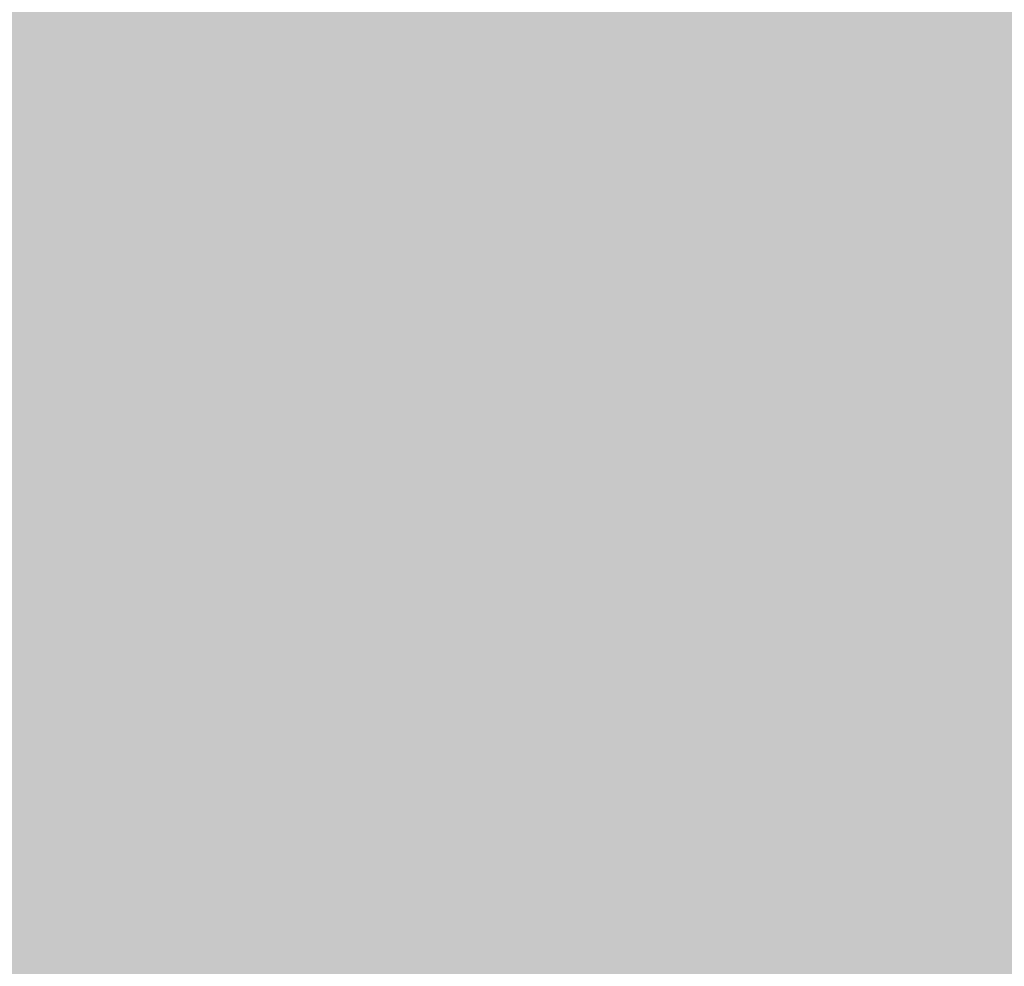
# Model space of a CAD drawing. Units: inches. Extents: x 2083 to 3317, y 1141 to 2115.
# Tile 137 of 256: x 3123.979 to 3126.132, y 1265.165 to 1267.234. Entities that reach past the tile are written whole.
import ezdxf

# ---------------------------------------------------------------- set-up
doc = ezdxf.new("R2010")
doc.units = ezdxf.units.IN
doc.layers.add('A-ANNO-DIMS', color=2, linetype='Continuous', lineweight=18)
doc.layers.add('A-WALL-PATT', color=251, linetype='Continuous', lineweight=13, true_color=0x636466)
doc.styles.get("Standard").update_dxf_attribs({"font": 'arial.ttf'})
doc.dimstyles.new('ISO-25', dxfattribs={"dimtxt": 12, "dimasz": 12, "dimexe": 1.25, "dimexo": 0.625, "dimtad": 1, "dimlunit": 3, "dimtxsty": 'Standard', "dimcen": 2.5, "dimadec": 0, "dimazin": 0, "dimtfac": 1, "dimtmove": 0, "dimatfit": 3, "dimfxl": 1, "dimarcsym": 0})

# ---------------------------------------------------------------- blocks, each defined once
blk = doc.blocks.new('*D26')
at = {"layer": 'A-ANNO-DIMS', "color": 0, "lineweight": -2, "transparency": 16777216}
for p, q in [((3088.9858, 1274.9151), (3088.9858, 1270.952)), ((3111.24, 1274.9151), (3111.24, 1270.952)), ((3076.9858, 1272.202), (2840.2624, 1272.202)), ((3111.24, 1272.202), (3088.9858, 1272.202)), ((3123.24, 1272.202), (3135.24, 1272.202))]:
    blk.add_line(p, q, dxfattribs=at)
at = {"layer": 'A-ANNO-DIMS', "color": 0, "transparency": 16777216}
for points in [[(3076.9858, 1274.202), (3076.9858, 1270.202), (3088.9858, 1272.202)], [(3123.24, 1274.202), (3123.24, 1270.202), (3111.24, 1272.202)]]:
    blk.add_solid(points, dxfattribs=at)
at = {"layer": 'Defpoints', "color": 0, "transparency": 16777216}
for p in [(3088.9858, 1275.5401), (3111.24, 1275.5401), (3088.9858, 1272.202)]:
    blk.add_point(p, dxfattribs=at)
at = {"layer": 'A-ANNO-DIMS', "color": 0, "transparency": 16777216, "insert": (2952.6241, 1279.0316), "char_height": 12, "attachment_point": 5}
blk.add_mtext('NIGHTSTAND 1\'-10 1/2" TYP.', dxfattribs=at)
blk = doc.blocks.new('*D27')
at = {"layer": 'A-ANNO-DIMS', "color": 0, "lineweight": -2, "transparency": 16777216}
for p, q in [((3114.5782, 1309.7943), (3114.5782, 1321.7943)), ((3111.865, 1297.7943), (3115.8282, 1297.7943)), ((3114.5782, 1297.7943), (3114.5782, 1275.5401)), ((3111.865, 1275.5401), (3115.8282, 1275.5401)), ((3114.5782, 1263.5401), (3114.5782, 1140.9886))]:
    blk.add_line(p, q, dxfattribs=at)
at = {"layer": 'A-ANNO-DIMS', "color": 0, "transparency": 16777216}
for points in [[(3112.5782, 1309.7943), (3116.5782, 1309.7943), (3114.5782, 1297.7943)], [(3112.5782, 1263.5401), (3116.5782, 1263.5401), (3114.5782, 1275.5401)]]:
    blk.add_solid(points, dxfattribs=at)
at = {"layer": 'Defpoints', "color": 0, "transparency": 16777216}
for p in [(3111.24, 1297.7943), (3111.24, 1275.5401), (3114.5782, 1275.5401)]:
    blk.add_point(p, dxfattribs=at)
at = {"layer": 'A-ANNO-DIMS', "color": 0, "transparency": 16777216, "insert": (3107.7485, 1196.2643), "char_height": 12, "attachment_point": 5, "rotation": 90}
blk.add_mtext('1\'-10 1/2" TYP.', dxfattribs=at)

msp = doc.modelspace()

# ---------------------------------------------------------------- hatches: boundary and pattern name
at = {"layer": 'A-WALL-PATT'}
h = msp.add_hatch(color=256, dxfattribs=at)
h.dxf.hatch_style = 1
h.paths.add_polyline_path([(3126.9598, 2020.7614), (2748.9598, 2020.7614), (2604.9598, 2020.7614), (2226.9598, 2020.7614), (2226.9598, 1702.7614), (2466.9598, 1702.7614), (2466.9598, 1582.7614), (2418.9598, 1582.7614), (2418.9598, 1477.7614), (2226.9598, 1477.7614), (2226.9598, 1263.2614), (2544.9598, 1263.2614), (2544.9598, 1411.7614), (2604.9598, 1411.7614), (2685.9598, 1411.7614), (2685.9598, 1420.7614), (2604.9598, 1420.7614), (2604.9598, 1573.7614), (2604.9598, 1702.7614), (2604.9598, 2011.7614), (2748.9598, 2011.7614), (2748.9598, 1702.7614), (2862.9598, 1702.7614), (2862.9598, 1621.7614), (2871.9598, 1621.7614), (2871.9598, 1702.7614), (2883.9598, 1702.7614), (2883.9598, 1706.9395, -0.026459), (2883.9598, 1711.7614), (2757.9598, 1711.7614), (2757.9598, 1807.7614), (2787.9598, 1807.7614), (2787.9598, 1812.2614), (2757.9598, 1812.2614), (2757.9598, 2011.7614), (2877.9598, 2011.7614), (2877.9598, 1812.2614), (2847.9598, 1812.2614), (2847.9598, 1807.7614), (2889.8357, 1807.7614), (2889.8357, 1812.2614), (2882.4598, 1812.2614), (2882.4598, 2011.7614), (3117.9598, 2011.7614), (3117.9598, 1812.2614), (2937.8357, 1812.2614), (2937.8357, 1807.7614), (2995.7098, 1807.7614), (2995.7098, 1796.1177), (3000.2098, 1796.1177), (3000.2098, 1807.7614), (3117.9598, 1807.7614), (3117.9598, 1711.7614), (3000.2098, 1711.7614), (3000.2098, 1760.1177), (2998.5727, 1760.1177, -0.020711), (2995.7098, 1760.1177), (2995.7098, 1711.7614), (2931.9598, 1711.7614), (2931.9598, 1702.7614), (3126.9598, 1702.7614)])
h.paths.add_polyline_path([(2471.4598, 2011.7614), (2471.4598, 1810.0114), (2462.7169, 1810.0114), (2462.7169, 1805.5114), (2505.9598, 1805.5114), (2505.9598, 1810.0114), (2475.9598, 1810.0114), (2475.9598, 2011.7614), (2595.9598, 2011.7614), (2595.9598, 1810.0114), (2565.9598, 1810.0114), (2565.9598, 1805.5114), (2595.9598, 1805.5114), (2595.9598, 1711.7614), (2235.9598, 1711.7614), (2235.9598, 1805.5114), (2353.7098, 1805.5114), (2353.7098, 1796.0542), (2358.2098, 1796.0542), (2358.2098, 1805.5114), (2414.7169, 1805.5114), (2414.7169, 1810.0114), (2235.9598, 1810.0114), (2235.9598, 2011.7614)], flags=16)
h.paths.add_polyline_path([(2270.2047, 1994.61), (2270.2047, 1970.61), (2246.2047, 1970.61), (2246.2047, 1994.61)], flags=0)
edge = h.paths.add_edge_path(flags=0)
edge.add_ellipse((2332.0274, 1899.7982), major_axis=(-3.043, 3.043), ratio=0.168252, start_angle=-161.3322, end_angle=-156.3071, ccw=False)
edge.add_ellipse((2333.082, 1898.7435), major_axis=(-1.0546, 1.0546), ratio=0.453532, start_angle=-123.371, end_angle=-94.1591)
edge = h.paths.add_edge_path(flags=0)
edge.add_ellipse((2332.0274, 1968.8763), major_axis=(3.043, 3.043), ratio=0.168252, start_angle=18.6678, end_angle=23.6929)
edge.add_spline(control_points=[(2332.9256, 1970.6911), (2332.2268, 1970.3361), (2330.8937, 1969.6589), (2328.4131, 1970.9321), (2327.2039, 1967.7487), (2324.7096, 1969.9556), (2322.5328, 1967.0124), (2320.0128, 1971.2958), (2317.6803, 1968.1578), (2316.0405, 1967.102), (2315.4269, 1966.8096)], knot_values=[0, 0, 0, 0, 2.267059, 4.324559, 6.685584, 8.878641, 11.121502, 14.300359, 17.755284, 19.732645, 19.732645, 19.732645, 19.732645], degree=3, periodic=0)
edge.add_ellipse((2332.0274, 1968.8763), major_axis=(3.043, 3.043), ratio=0.168252, start_angle=18.6678, end_angle=23.6929, ccw=False)
edge.add_ellipse((2333.082, 1969.9309), major_axis=(1.0546, 1.0546), ratio=0.453532, start_angle=56.629, end_angle=85.8409, ccw=False)
edge = h.paths.add_edge_path(flags=0)
edge.add_spline(control_points=[(2296.4283, 1967.9879), (2293.6278, 1965.3363), (2287.7036, 1959.7271), (2299.7439, 1949.9957), (2294.5326, 1935.6685), (2290.5732, 1920.6035), (2293.3941, 1909.9737), (2296.1854, 1904.9665)], knot_values=[0.099185, 0.099185, 0.099185, 0.099185, 0.345301, 0.619822, 0.982653, 1.386093, 1.810555, 1.810555, 1.810555, 1.810555], degree=3, periodic=0)
edge.add_spline(control_points=[(2296.1854, 1904.9665), (2297.3836, 1902.6193), (2298.001, 1901.9493), (2298.553, 1901.4682)], knot_values=[0.006246, 0.006246, 0.006246, 0.006246, 0.055476, 0.055476, 0.055476, 0.055476], degree=3, periodic=0)
edge.add_spline(control_points=[(2298.553, 1901.4682), (2297.2586, 1900.9232), (2295.2253, 1900.2321), (2293.0602, 1900.6142), (2292.1014, 1900.7884), (2292.0896, 1900.7906)], knot_values=[0.312835, 0.312835, 0.312835, 0.312835, 0.40178, 0.474987, 0.475903, 0.475903, 0.475903, 0.475903], degree=3, periodic=0)
edge.add_arc((2292.7936, 1904.6641), 3.937, 215.4209, 259.6982, ccw=False)
edge.add_spline(control_points=[(2289.5853, 1902.3823), (2289.4767, 1902.5351), (2289.3685, 1902.688), (2289.2609, 1902.8412)], knot_values=[0.102872, 0.102872, 0.102872, 0.102872, 0.116896, 0.116896, 0.116896, 0.116896], degree=3, periodic=0)
edge.add_spline(control_points=[(2289.2609, 1902.8412), (2288.6866, 1902.5502), (2287.64, 1902.0199), (2285.8813, 1901.874), (2283.853, 1901.5044), (2281.72, 1899.7105), (2278.467, 1899.4929), (2276.1571, 1901.8832), (2272.259, 1899.8041), (2267.7776, 1901.8432), (2262.2439, 1900.184), (2257.4149, 1901.7821), (2254.3184, 1900.7261), (2253.1783, 1900.3373)], knot_values=[0, 0, 0, 0, 1.907977, 3.477176, 5.261074, 7.972851, 11.680248, 13.717921, 16.939592, 22.789562, 27.502503, 33.595215, 37.145618, 37.145618, 37.145618, 37.145618], degree=3, periodic=0)
edge.add_line((2253.1783, 1900.3373), (2250.2442, 1902.8412))
edge.add_line((2250.2442, 1902.8412), (2250.2442, 1965.8333))
edge.add_line((2250.2442, 1965.8333), (2253.1783, 1968.3371))
edge.add_spline(control_points=[(2253.1783, 1968.3371), (2254.3184, 1967.9483), (2257.4149, 1966.8924), (2262.2439, 1968.4904), (2267.7776, 1966.8313), (2271.5267, 1968.5372), (2273.8759, 1967.8283), (2274.2067, 1967.7276)], knot_values=[0, 0, 0, 0, 0.09018, 0.244935, 0.364644, 0.513233, 0.537855, 0.537855, 0.537855, 0.537855], degree=3, periodic=0)
edge.add_arc((2274.3529, 1963.7933), 3.937, 72.0511, 92.1279, ccw=False)
edge.add_arc((2281.2969, 1985.23), 18.5963, 252.05113, 288.56572)
edge.add_arc((2292.3167, 1956.0289), 12.6461, 71.02679, 113.77822, ccw=False)
edge = h.paths.add_edge_path(flags=0)
edge.add_spline(control_points=[(2274.8994, 1951.8562), (2275.0662, 1951.6166), (2275.2327, 1951.3766), (2275.398, 1951.1359)], knot_values=[1.409916, 1.409916, 1.409916, 1.409916, 1.43159, 1.43159, 1.43159, 1.43159], degree=3, periodic=0)
edge.add_spline(control_points=[(2275.398, 1951.1359), (2275.7921, 1950.5619), (2276.1792, 1949.9838), (2276.5455, 1949.3971)], knot_values=[1.358238, 1.358238, 1.358238, 1.358238, 1.409916, 1.409916, 1.409916, 1.409916], degree=3, periodic=0)
edge.add_line((2276.5455, 1949.3971), (2277.4373, 1947.8622))
edge.add_spline(control_points=[(2277.4373, 1947.8622), (2276.3038, 1945.6731), (2274.6397, 1942.4269), (2274.6316, 1938.0939), (2272.7991, 1930.8515), (2274.3564, 1943.897), (2275.9477, 1947.9234), (2276.5455, 1949.3971)], knot_values=[0.005632, 0.005632, 0.005632, 0.005632, 0.186014, 0.266002, 0.357087, 0.59639, 0.739732, 0.739732, 0.739732, 0.739732], degree=3, periodic=0)
edge.add_spline(control_points=[(2276.5455, 1949.3971), (2276.1792, 1949.9838), (2275.7921, 1950.5619), (2275.398, 1951.1359)], knot_values=[1.358238, 1.358238, 1.358238, 1.358238, 1.409916, 1.409916, 1.409916, 1.409916], degree=3, periodic=0)
edge.add_spline(control_points=[(2275.398, 1951.1359), (2274.9425, 1950.0805), (2274.2078, 1948.0253), (2273.9346, 1944.8515), (2272.4685, 1937.6275), (2273.4662, 1945.6965), (2274.7006, 1951.0595), (2274.8994, 1951.8562)], knot_values=[0.104364, 0.104364, 0.104364, 0.104364, 0.189636, 0.269624, 0.36071, 0.600013, 0.644622, 0.644622, 0.644622, 0.644622], degree=3, periodic=0)
h.paths.add_polyline_path([(2269.1675, 1963.1276, -0.357527), (2268.1706, 1960.9764, -0.092561), (2268.1706, 1939.4363, -0.357527), (2269.1675, 1937.2851, -0.357527), (2267.0163, 1938.282, -0.164785), (2254.6856, 1938.282, -0.357527), (2252.5344, 1937.2851, -0.357527), (2253.5313, 1939.4363, -0.092561), (2253.5313, 1960.9764, -0.357527), (2252.5344, 1963.1276, -0.357527), (2254.6856, 1962.1307, -0.164785), (2267.0163, 1962.1307, -0.357527)], flags=0)
h.paths.add_polyline_path([(2248.8741, 1967.8018), (2248.8741, 1957.0277), (2249.4578, 1957.0277), (2249.4578, 1911.6468), (2248.8741, 1911.6468), (2248.8741, 1900.8727), (2246.5119, 1900.8727, 0.197327), (2244.1497, 1902.4569), (2244.1497, 1966.2176, 0.197327), (2246.5119, 1967.8018)], flags=0)
h.paths.add_polyline_path([(2269.1675, 1931.3893, -0.357527), (2268.1706, 1929.2381, -0.092561), (2268.1706, 1907.6981, -0.357527), (2269.1675, 1905.5469, -0.357527), (2267.0163, 1906.5438, -0.164785), (2254.6856, 1906.5438, -0.357527), (2252.5344, 1905.5469, -0.357527), (2253.5313, 1907.6981, -0.092561), (2253.5313, 1929.2381, -0.357527), (2252.5344, 1931.3893, -0.357527), (2254.6856, 1930.3925, -0.164785), (2267.0163, 1930.3925, -0.357527)], flags=0)
edge = h.paths.add_edge_path(flags=0)
edge.add_spline(control_points=[(2276.1969, 1906.7237), (2276.1681, 1909.0289), (2276.114, 1913.3719), (2270.5984, 1924.925), (2273.9052, 1919.0128), (2275.9217, 1916.2621), (2275.4746, 1912.4021), (2277.2579, 1910.3806), (2276.696, 1908.225), (2276.6462, 1906.813), (2276.6178, 1906.0084)], knot_values=[0, 0, 0, 0, 8.61026, 16.221274, 18.843057, 23.804898, 27.440828, 29.356102, 31.203478, 33.650687, 33.650687, 33.650687, 33.650687], degree=3, periodic=0)
edge.add_spline(control_points=[(2276.6178, 1906.0084), (2276.6233, 1905.6241), (2276.4977, 1904.6287), (2275.4418, 1903.8547), (2274.9373, 1903.0804), (2274.8591, 1902.8412)], knot_values=[0.156488, 0.156488, 0.156488, 0.156488, 0.184398, 0.231376, 0.250598, 0.250598, 0.250598, 0.250598], degree=3, periodic=0)
edge.add_line((2274.8591, 1902.8412), (2276.506, 1902.8412))
edge.add_spline(control_points=[(2276.506, 1902.8412), (2276.7883, 1903.0849), (2277.6651, 1904.1252), (2278.2495, 1904.3407), (2277.6539, 1908.5274), (2278.1557, 1906.2278), (2278.1005, 1905.2859), (2278.8467, 1904.069), (2277.8568, 1903.4149), (2277.8742, 1902.991), (2277.9036, 1902.8412)], knot_values=[0.059574, 0.059574, 0.059574, 0.059574, 0.080753, 0.103741, 0.16972, 0.176036, 0.207137, 0.240474, 0.262341, 0.27366, 0.27366, 0.27366, 0.27366], degree=3, periodic=0)
edge.add_line((2277.9036, 1902.8412), (2280.0298, 1902.8412))
edge.add_spline(control_points=[(2280.0298, 1902.8412), (2279.8882, 1903.0884), (2279.4993, 1903.9816), (2280.1523, 1905.9393), (2278.1036, 1909.6578), (2279.7624, 1907.1853), (2280.3279, 1904.8749), (2280.4851, 1903.4896), (2281.4633, 1903.2494), (2281.7583, 1902.9365), (2281.834, 1902.8412)], knot_values=[0.013856, 0.013856, 0.013856, 0.013856, 0.034874, 0.088867, 0.107879, 0.126738, 0.158714, 0.193757, 0.217487, 0.226722, 0.226722, 0.226722, 0.226722], degree=3, periodic=0)
edge.add_spline(control_points=[(2281.834, 1902.8412), (2281.7875, 1902.8267), (2281.647, 1902.783), (2281.3955, 1902.8595), (2281.0881, 1902.9852), (2280.7207, 1903.0609), (2280.3335, 1903.0257), (2280.1248, 1902.8989), (2280.0298, 1902.8412)], knot_values=[0, 0, 0, 0, 0.14413, 0.435517, 0.749276, 1.153046, 1.548371, 1.878348, 1.878348, 1.878348, 1.878348], degree=3, periodic=0)
edge.add_line((2280.0298, 1902.8412), (2277.9036, 1902.8412))
edge.add_spline(control_points=[(2277.9036, 1902.8412), (2277.8929, 1902.7959), (2277.8654, 1902.6796), (2277.6075, 1902.6875), (2277.2741, 1902.8007), (2276.8379, 1902.6198), (2276.5838, 1902.7893), (2276.506, 1902.8412)], knot_values=[0, 0, 0, 0, 0.127189, 0.326199, 0.628009, 1.24357, 1.515331, 1.515331, 1.515331, 1.515331], degree=3, periodic=0)
edge.add_line((2276.506, 1902.8412), (2274.8591, 1902.8412))
edge.add_spline(control_points=[(2274.8591, 1902.8412), (2274.8144, 1902.8986), (2274.7251, 1903.0134), (2274.4935, 1903.119), (2274.2443, 1902.9605), (2273.9371, 1903.1849), (2273.614, 1902.9831), (2273.4083, 1902.883), (2273.3223, 1902.8412)], knot_values=[0, 0, 0, 0, 0.21843, 0.436957, 0.687977, 0.990379, 1.398396, 1.69185, 1.69185, 1.69185, 1.69185], degree=3, periodic=0)
edge.add_spline(control_points=[(2273.3223, 1902.8412), (2273.6167, 1903.4457), (2274.274, 1904.5383), (2276.0272, 1904.5737), (2276.207, 1906.5836), (2276.1969, 1906.7237)], knot_values=[0.012227, 0.012227, 0.012227, 0.012227, 0.059472, 0.106218, 0.134458, 0.134458, 0.134458, 0.134458], degree=3, periodic=0)
h.paths.add_polyline_path([(2270.7761, 1897.7898), (2270.7761, 1873.7898), (2246.7761, 1873.7898), (2246.7761, 1897.7898)], flags=0)
h.paths.add_polyline_path([(2353.7098, 1760.0051), (2353.7098, 1760.0542), (2358.2098, 1760.0542, -0.033729)], flags=0)
h.paths.add_polyline_path([(2321.8191, 1737.5292), (2341.9953, 1737.5292, -0.414214), (2343.2033, 1736.3212), (2343.2033, 1721.0206, -0.414214), (2341.9953, 1719.8127), (2321.8191, 1719.8127, -0.414214), (2320.6112, 1721.0206), (2320.6112, 1736.3212, -0.414214)], flags=0)
h.paths.add_polyline_path([(2324.235, 1736.3212), (2339.5794, 1736.3212, -0.414214), (2341.9953, 1733.9053), (2341.9953, 1725.4497, -0.414214), (2339.5794, 1723.0338), (2333.6806, 1723.0338), (2333.8453, 1722.0455, -0.870646), (2335.4254, 1721.8259, -0.767327), (2333.9227, 1721.4232), (2331.291, 1721.4232, -0.767327), (2329.7883, 1721.8259, -0.870646), (2331.3684, 1722.0455), (2331.5331, 1723.0338), (2324.235, 1723.0338, -0.414214), (2321.8191, 1725.4497), (2321.8191, 1733.9053, -0.414214)], flags=0)
h.paths.add_polyline_path([(2570.4838, 1928.6154), (2589.6838, 1928.6154), (2590.1688, 1928.6154), (2590.1688, 1904.9934), (2570.4838, 1904.9934)], flags=0)
h.paths.add_polyline_path([(2574.4473, 1927.2638, -1), (2572.8288, 1927.2638, -1)], flags=0)
h.paths.add_polyline_path([(2573.0899, 1926.9409), (2573.925, 1927.776), (2574.1477, 1927.5533), (2573.3126, 1926.7182)], flags=0)
h.paths.add_polyline_path([(2578.7791, 1919.7296, -1), (2571.5917, 1919.7296, -1)], flags=0)
h.paths.add_polyline_path([(2578.3854, 1919.7296, -1), (2571.9854, 1919.7296, -1)], flags=0)
h.paths.add_polyline_path([(2331.5958, 1729.4762, -1), (2333.618, 1729.4762, -1)], flags=0)
h.paths.add_polyline_path([(2578.0342, 1927.2638, -1), (2576.4157, 1927.2638, -1)], flags=0)
h.paths.add_polyline_path([(2576.6889, 1927.5311), (2576.9116, 1927.7538), (2577.7467, 1926.9186), (2577.524, 1926.6959)], flags=0)
h.paths.add_polyline_path([(2578.1391, 1909.8595, -1), (2572.2317, 1909.8595, -1)], flags=0)
h.paths.add_polyline_path([(2577.7454, 1909.8595, -1), (2572.6254, 1909.8595, -1)], flags=0)
h.paths.add_polyline_path([(2583.7977, 1927.2638, -1), (2582.1792, 1927.2638, -1)], flags=0)
h.paths.add_polyline_path([(2582.7186, 1927.7538), (2583.5538, 1926.9186), (2583.3311, 1926.6959), (2582.4959, 1927.5311)], flags=0)
h.paths.add_polyline_path([(2582.4959, 1927.5311), (2582.7186, 1927.7538), (2583.5538, 1926.9186), (2583.3311, 1926.6959)], flags=0)
h.paths.add_polyline_path([(2587.7391, 1920.5296, -1), (2581.8317, 1920.5296, -1)], flags=0)
h.paths.add_polyline_path([(2587.3454, 1920.5296, -1), (2582.2254, 1920.5296, -1)], flags=0)
h.paths.add_polyline_path([(2587.3846, 1927.2638, -1), (2585.7661, 1927.2638, -1)], flags=0)
h.paths.add_polyline_path([(2586.082, 1926.9802), (2586.9172, 1927.8154), (2587.1399, 1927.5927), (2586.3047, 1926.7575)], flags=0)
h.paths.add_polyline_path([(2588.3791, 1910.6595, -1), (2581.1917, 1910.6595, -1)], flags=0)
h.paths.add_polyline_path([(2587.9854, 1910.6595, -1), (2581.5854, 1910.6595, -1)], flags=0)
h.paths.add_polyline_path([(2417.1677, 1729.4779), (2437.3439, 1729.4779, -0.414214), (2438.5519, 1728.2699), (2438.5519, 1712.9693, -0.414214), (2437.3439, 1711.7614), (2417.1677, 1711.7614, -0.414214), (2415.9598, 1712.9693), (2415.9598, 1728.2699, -0.414214)], flags=0)
h.paths.add_polyline_path([(2419.5836, 1728.2699), (2434.928, 1728.2699, -0.414214), (2437.3439, 1725.8541), (2437.3439, 1717.3984, -0.414214), (2434.928, 1714.9825), (2429.0292, 1714.9825), (2429.1939, 1713.9942, -0.870646), (2430.774, 1713.7746, -0.767327), (2429.2713, 1713.372), (2426.6396, 1713.372, -0.767327), (2425.1369, 1713.7746, -0.870646), (2426.717, 1713.9942), (2426.8817, 1714.9825), (2419.5836, 1714.9825, -0.414214), (2417.1677, 1717.3984), (2417.1677, 1725.8541, -0.414214)], flags=0)
h.paths.add_polyline_path([(2419.5836, 1728.2699), (2434.928, 1728.2699, -0.414214), (2437.3439, 1725.8541), (2437.3439, 1717.3984, -0.414214), (2434.928, 1714.9825), (2429.0292, 1714.9825), (2428.3581, 1719.009), (2427.5528, 1719.009), (2426.8817, 1714.9825), (2419.5836, 1714.9825, -0.414214), (2417.1677, 1717.3984), (2417.1677, 1725.8541, -0.414214)], flags=0)
h.paths.add_polyline_path([(2426.9444, 1721.4249, -1), (2428.9666, 1721.4249, -1)], flags=0)
h.paths.add_polyline_path([(2475.9598, 1702.7614), (2595.9598, 1702.7614), (2595.9598, 1582.7614), (2475.9598, 1582.7614)], flags=16)
h.paths.add_polyline_path([(2427.9598, 1573.7614), (2595.9598, 1573.7614), (2595.9598, 1468.7614), (2595.9598, 1420.7614), (2384.4598, 1420.7614), (2384.4598, 1468.7614), (2427.9598, 1468.7614)], flags=16)
h.paths.add_polyline_path([(2379.9598, 1468.7614), (2379.9598, 1420.7614), (2235.9598, 1420.7614), (2235.9598, 1468.7614)], flags=16)
h.paths.add_polyline_path([(2317.816, 1466.6958), (2337.9922, 1466.6958, -0.414214), (2339.2002, 1465.4878), (2339.2002, 1450.1872, -0.414214), (2337.9922, 1448.9792), (2317.816, 1448.9792, -0.414214), (2316.6081, 1450.1872), (2316.6081, 1465.4878, -0.414214)], flags=0)
h.paths.add_polyline_path([(2320.2319, 1465.4878), (2335.5763, 1465.4878, -0.414214), (2337.9922, 1463.0719), (2337.9922, 1454.6163, -0.414214), (2335.5763, 1452.2004), (2329.6775, 1452.2004), (2329.8422, 1451.212, -0.870646), (2331.4223, 1450.9925, -0.767327), (2329.9196, 1450.5898), (2327.2879, 1450.5898, -0.767327), (2325.7852, 1450.9925, -0.870646), (2327.3653, 1451.212), (2327.53, 1452.2004), (2320.2319, 1452.2004, -0.414214), (2317.816, 1454.6163), (2317.816, 1463.0719, -0.414214)], flags=0)
h.paths.add_polyline_path([(2320.2319, 1465.4878), (2335.5763, 1465.4878, -0.414214), (2337.9922, 1463.0719), (2337.9922, 1454.6163, -0.414214), (2335.5763, 1452.2004), (2329.6775, 1452.2004), (2329.0064, 1456.2269), (2328.2011, 1456.2269), (2327.53, 1452.2004), (2320.2319, 1452.2004, -0.414214), (2317.816, 1454.6163), (2317.816, 1463.0719, -0.414214)], flags=0)
h.paths.add_polyline_path([(2327.5926, 1458.6428, -1), (2329.6148, 1458.6428, -1)], flags=0)
h.paths.add_polyline_path([(2244.4117, 1433.3405), (2241.9209, 1433.3405, -0.414214), (2240.0179, 1435.2435), (2240.0179, 1440.9528, -0.414211), (2241.9209, 1442.8559), (2244.4117, 1442.8559, -1.976472)], flags=0)
h.paths.add_polyline_path([(2245.3569, 1434.3975, -0.414214), (2245.3569, 1441.7988, -2.144098)], flags=0)
h.paths.add_polyline_path([(2535.9598, 1416.2614), (2535.9598, 1272.2614), (2235.9598, 1272.2614), (2235.9598, 1416.2614)], flags=16)
h.paths.add_polyline_path([(2260.1196, 1384.2928), (2260.1196, 1362.0386), (2237.8654, 1362.0386), (2237.8654, 1384.2928)], flags=0)
edge = h.paths.add_edge_path(flags=0)
edge.add_line((2318.2518, 1362.0933), (2318.1458, 1362.001))
edge.add_ellipse((2317.4451, 1360.431), major_axis=(2.8216, 2.8216), ratio=0.168252, start_angle=18.6678, end_angle=20.9481, ccw=False)
edge.add_ellipse((2318.423, 1361.409), major_axis=(0.9779, 0.9779), ratio=0.453532, start_angle=56.629, end_angle=70.2262, ccw=False)
edge = h.paths.add_edge_path(flags=0)
edge.add_line((2319.1074, 1295.5711), (2319.015, 1295.6771))
edge.add_ellipse((2317.4451, 1296.3778), major_axis=(-2.8216, 2.8216), ratio=0.168252, start_angle=-161.3322, end_angle=-159.0519, ccw=False)
edge.add_ellipse((2318.423, 1295.3999), major_axis=(-0.9779, 0.9779), ratio=0.453532, start_angle=-123.371, end_angle=-109.7738)
edge = h.paths.add_edge_path(flags=0)
edge.add_spline(control_points=[(2284.2103, 1301.1702), (2284.5807, 1300.4447), (2284.8912, 1299.892), (2285.1596, 1299.461)], knot_values=[0.039066, 0.039066, 0.039066, 0.039066, 0.055476, 0.055476, 0.055476, 0.055476], degree=3, periodic=0)
edge.add_line((2285.1596, 1299.461), (2284.2103, 1301.1702))
edge = h.paths.add_edge_path(flags=0)
edge.add_line((2280.4125, 1297.298), (2283.37, 1297.0361))
edge.add_line((2283.37, 1297.0361), (2286.4057, 1297.9263))
edge.add_spline(control_points=[(2286.4057, 1297.9263), (2285.3055, 1297.4631), (2284.3448, 1297.1292), (2283.37, 1297.0361)], knot_values=[0.394369, 0.394369, 0.394369, 0.394369, 0.475903, 0.475903, 0.475903, 0.475903], degree=3, periodic=0)
edge.add_spline(control_points=[(2283.37, 1297.0361), (2283.2814, 1297.0277), (2282.3163, 1296.9573), (2281.3125, 1297.1345), (2280.4234, 1297.296), (2280.4125, 1297.298)], knot_values=[0.312835, 0.312835, 0.312835, 0.312835, 0.320246, 0.393453, 0.394369, 0.394369, 0.394369, 0.394369], degree=3, periodic=0)
edge = h.paths.add_edge_path(flags=0)
edge.add_line((2284.4356, 1359.6073), (2280.4463, 1355.328))
edge.add_line((2280.4463, 1355.328), (2279.58, 1351.0178))
edge.add_line((2279.58, 1351.0178), (2282.413, 1346.5804))
edge.add_spline(control_points=[(2282.413, 1346.5804), (2283.1533, 1345.5892), (2284.2529, 1344.0289), (2284.801, 1342.3872), (2284.9352, 1341.8055)], knot_values=[1.240098, 1.240098, 1.240098, 1.240098, 1.332892, 1.382712, 1.382712, 1.382712, 1.382712], degree=3, periodic=0)
edge.add_spline(control_points=[(2284.9352, 1341.8055), (2285.3191, 1340.1406), (2285.233, 1338.4092), (2284.9099, 1336.6541)], knot_values=[1.097484, 1.097484, 1.097484, 1.097484, 1.240098, 1.240098, 1.240098, 1.240098], degree=3, periodic=0)
edge.add_spline(control_points=[(2284.9099, 1336.6541), (2284.5868, 1334.899), (2284.0267, 1333.1203), (2283.4626, 1331.3606)], knot_values=[0.95487, 0.95487, 0.95487, 0.95487, 1.097484, 1.097484, 1.097484, 1.097484], degree=3, periodic=0)
edge.add_line((2283.4626, 1331.3606), (2281.8904, 1326.1534))
edge.add_line((2281.8904, 1326.1534), (2280.7563, 1321.0561))
edge.add_line((2280.7563, 1321.0561), (2280.2992, 1316.002))
edge.add_line((2280.2992, 1316.002), (2280.7159, 1310.9501))
edge.add_line((2280.7159, 1310.9501), (2282.0281, 1305.9721))
edge.add_line((2282.0281, 1305.9721), (2284.2103, 1301.1702))
edge.add_spline(control_points=[(2284.2103, 1301.1702), (2283.3407, 1302.7302), (2282.6119, 1304.3365), (2282.0281, 1305.9721)], knot_values=[0.099185, 0.099185, 0.099185, 0.099185, 0.241799, 0.241799, 0.241799, 0.241799], degree=3, periodic=0)
edge.add_spline(control_points=[(2282.0281, 1305.9721), (2281.4443, 1307.6078), (2281.0055, 1309.2728), (2280.7159, 1310.9501)], knot_values=[0.241799, 0.241799, 0.241799, 0.241799, 0.384413, 0.384413, 0.384413, 0.384413], degree=3, periodic=0)
edge.add_spline(control_points=[(2280.7159, 1310.9501), (2280.4332, 1312.5876), (2280.2894, 1314.277), (2280.2989, 1315.962), (2280.2992, 1316.002)], knot_values=[0.384413, 0.384413, 0.384413, 0.384413, 0.523647, 0.527028, 0.527028, 0.527028, 0.527028], degree=3, periodic=0)
edge.add_spline(control_points=[(2280.2992, 1316.002), (2280.3123, 1317.687), (2280.4779, 1319.3679), (2280.7563, 1321.0561)], knot_values=[0.527028, 0.527028, 0.527028, 0.527028, 0.669642, 0.669642, 0.669642, 0.669642], degree=3, periodic=0)
edge.add_spline(control_points=[(2280.7563, 1321.0561), (2281.0346, 1322.7443), (2281.4259, 1324.4396), (2281.8904, 1326.1534)], knot_values=[0.669642, 0.669642, 0.669642, 0.669642, 0.812256, 0.812256, 0.812256, 0.812256], degree=3, periodic=0)
edge.add_spline(control_points=[(2281.8904, 1326.1534), (2282.2644, 1327.5333), (2282.7879, 1329.2618), (2283.3528, 1331.0178), (2283.4626, 1331.3606)], knot_values=[0.812256, 0.812256, 0.812256, 0.812256, 0.927087, 0.95487, 0.95487, 0.95487, 0.95487], degree=3, periodic=0)
edge.add_line((2283.4626, 1331.3606), (2284.9099, 1336.6541))
edge.add_line((2284.9099, 1336.6541), (2284.9352, 1341.8055))
edge.add_line((2284.9352, 1341.8055), (2282.413, 1346.5804))
edge.add_spline(control_points=[(2282.413, 1346.5804), (2281.2751, 1348.1038), (2280.0784, 1349.5703), (2279.58, 1351.0178)], knot_values=[1.382712, 1.382712, 1.382712, 1.382712, 1.525326, 1.525326, 1.525326, 1.525326], degree=3, periodic=0)
edge.add_spline(control_points=[(2279.58, 1351.0178), (2279.4433, 1351.4147), (2279.1363, 1352.8569), (2279.7352, 1354.2904), (2280.4463, 1355.328)], knot_values=[1.525326, 1.525326, 1.525326, 1.525326, 1.564439, 1.667941, 1.667941, 1.667941, 1.667941], degree=3, periodic=0)
edge.add_spline(control_points=[(2280.4463, 1355.328), (2281.4261, 1356.7578), (2282.9308, 1358.1826), (2284.4356, 1359.6073)], knot_values=[1.667941, 1.667941, 1.667941, 1.667941, 1.810555, 1.810555, 1.810555, 1.810555], degree=3, periodic=0)
edge.add_arc((2280.6231, 1348.5182), 11.7262, 71.02679, 113.77822)
edge.add_arc((2270.4049, 1375.5952), 17.2436, 252.05113, 288.56572, ccw=False)
edge.add_arc((2263.966, 1355.7178), 3.6506, 72.0511, 92.1279)
edge.add_arc((2263.966, 1355.7178), 3.6506, 92.1279, 177.9851)
edge.add_spline(control_points=[(2260.3176, 1355.8462), (2260.2604, 1354.2207), (2260.5513, 1350.1865), (2262.9993, 1346.7663), (2264.4727, 1344.649)], knot_values=[1.43159, 1.43159, 1.43159, 1.43159, 1.564144, 1.770695, 1.770695, 1.770695, 1.770695], degree=3, periodic=0)
edge.add_line((2264.4727, 1344.649), (2264.9356, 1343.9825))
edge.add_spline(control_points=[(2263.801, 1340.2481), (2263.8432, 1340.5141), (2264.0672, 1341.7565), (2264.5127, 1343.0025), (2264.935, 1343.9811)], knot_values=[0.53657, 0.53657, 0.53657, 0.53657, 0.559349, 0.644622, 0.644622, 0.644622, 0.644622], degree=3, periodic=0)
edge.add_spline(control_points=[(2264.935, 1343.9811), (2265.1178, 1343.715), (2265.2989, 1343.4479), (2265.4768, 1343.1794)], knot_values=[1.384077, 1.384077, 1.384077, 1.384077, 1.409916, 1.409916, 1.409916, 1.409916], degree=3, periodic=0)
edge.add_spline(control_points=[(2265.4768, 1343.1794), (2265.6546, 1342.9108), (2265.8293, 1342.6408), (2265.9991, 1342.3688)], knot_values=[1.358238, 1.358238, 1.358238, 1.358238, 1.384077, 1.384077, 1.384077, 1.384077], degree=3, periodic=0)
edge.add_line((2265.9991, 1342.3688), (2266.826, 1340.9455))
edge.add_spline(control_points=[(2266.826, 1340.9455), (2268.8944, 1337.0897), (2271.3982, 1325.843), (2270.5162, 1310.5686), (2275.9194, 1301.8606), (2277.7895, 1299.1994)], knot_values=[0.116896, 0.116896, 0.116896, 0.116896, 0.472987, 1.050969, 1.313793, 1.313793, 1.313793, 1.313793], degree=3, periodic=0)
edge.add_spline(control_points=[(2277.7895, 1299.1994), (2277.8394, 1299.1285), (2277.8894, 1299.0575), (2277.9396, 1298.9866)], knot_values=[0.109884, 0.109884, 0.109884, 0.109884, 0.116896, 0.116896, 0.116896, 0.116896], degree=3, periodic=0)
edge.add_line((2277.9396, 1298.9866), (2277.7888, 1299.1991))
edge.add_spline(control_points=[(2277.7888, 1299.1991), (2277.2566, 1298.9294), (2276.2864, 1298.4379), (2275.0394, 1298.3344), (2274.3833, 1298.2389), (2274.2153, 1298.2093)], knot_values=[33.12187, 33.12187, 33.12187, 33.12187, 35.029056, 36.598255, 37.144827, 37.144827, 37.144827, 37.144827], degree=3, periodic=0)
edge.add_line((2274.2153, 1298.2093), (2273.0731, 1297.893))
edge.add_spline(control_points=[(2273.0731, 1297.893), (2272.3229, 1297.5798), (2271.0392, 1296.5105), (2269.2484, 1296.2261), (2268.4231, 1296.3747)], knot_values=[26.532584, 26.532584, 26.532584, 26.532584, 29.198919, 31.839101, 31.839101, 31.839101, 31.839101], degree=3, periodic=0)
edge.add_line((2268.4231, 1296.3747), (2263.8785, 1297.4575))
edge.add_spline(control_points=[(2263.8785, 1297.4575), (2263.5561, 1297.3594), (2261.8603, 1296.8387), (2260.2388, 1297.2824), (2258.9335, 1297.5165)], knot_values=[15.919551, 15.919551, 15.919551, 15.919551, 16.939592, 21.226067, 21.226067, 21.226067, 21.226067], degree=3, periodic=0)
edge.add_line((2258.9335, 1297.5165), (2254.0552, 1297.329))
edge.add_spline(control_points=[(2254.0552, 1297.329), (2253.7555, 1297.2958), (2252.1137, 1297.1652), (2250.4619, 1297.5442), (2249.1297, 1297.6679)], knot_values=[5.306517, 5.306517, 5.306517, 5.306517, 6.276435, 10.613034, 10.613034, 10.613034, 10.613034], degree=3, periodic=0)
edge.add_line((2249.1297, 1297.6679), (2244.3316, 1296.8778))
edge.add_line((2244.3316, 1296.8778), (2241.611, 1299.1994))
edge.add_line((2241.611, 1299.1994), (2241.611, 1357.6094))
edge.add_line((2241.611, 1357.6094), (2244.3316, 1359.9311))
edge.add_line((2244.3316, 1359.9311), (2252.7288, 1359.5427))
edge.add_spline(control_points=[(2252.7288, 1359.5427), (2252.8709, 1359.5464), (2253.3057, 1359.5482), (2253.7398, 1359.5143), (2254.0317, 1359.4824)], knot_values=[0.233291, 0.233291, 0.233291, 0.233291, 0.244935, 0.268927, 0.268927, 0.268927, 0.268927], degree=3, periodic=0)
edge.add_line((2254.0317, 1359.4824), (2259.5872, 1359.4164))
edge.add_spline(control_points=[(2259.5872, 1359.4164), (2260.6771, 1359.6285), (2262.0732, 1359.897), (2263.5237, 1359.4593), (2263.8304, 1359.366)], knot_values=[0.422516, 0.422516, 0.422516, 0.422516, 0.513233, 0.537855, 0.537855, 0.537855, 0.537855], degree=3, periodic=0)
edge.add_arc((2263.966, 1355.7178), 3.6506, 72.0511, 92.1279, ccw=False)
edge.add_arc((2270.4049, 1375.5952), 17.2436, 252.05113, 288.56572)
edge.add_arc((2280.6231, 1348.5182), 11.7262, 71.02679, 113.77822, ccw=False)
h.paths.add_polyline_path([(2240.3405, 1359.4347), (2240.3405, 1349.4444), (2240.8818, 1349.4444), (2240.8818, 1307.3645), (2240.3405, 1307.3645), (2240.3405, 1297.3741), (2238.1502, 1297.3741, 0.197327), (2235.9598, 1298.8431), (2235.9598, 1357.9657, 0.197327), (2238.1502, 1359.4347)], flags=0)
h.paths.add_polyline_path([(2259.1578, 1355.1005, -0.357527), (2258.2334, 1353.1058, -0.092561), (2258.2334, 1333.1326, -0.357527), (2259.1578, 1331.1379, -0.357527), (2257.1631, 1332.0622, -0.164785), (2245.7293, 1332.0622, -0.357527), (2243.7346, 1331.1379, -0.357527), (2244.6589, 1333.1326, -0.092561), (2244.6589, 1353.1058, -0.357527), (2243.7346, 1355.1005, -0.357527), (2245.7293, 1354.1761, -0.164785), (2257.1631, 1354.1761, -0.357527)], flags=0)
edge = h.paths.add_edge_path(flags=0)
edge.add_line((2265.9991, 1342.3688), (2266.826, 1340.9455))
edge.add_line((2266.826, 1340.9455), (2265.3076, 1337.8141))
edge.add_line((2265.3076, 1337.8141), (2264.3582, 1334.6529))
edge.add_line((2264.3582, 1334.6529), (2264.262, 1333.7997))
edge.add_spline(control_points=[(2264.262, 1333.7997), (2264.2084, 1333.1871), (2264.1621, 1332.3655), (2264.0071, 1331.4139), (2263.969, 1331.2018)], knot_values=[0.464444, 0.464444, 0.464444, 0.464444, 0.516691, 0.531608, 0.531608, 0.531608, 0.531608], degree=3, periodic=0)
edge.add_spline(control_points=[(2263.969, 1331.2018), (2263.7745, 1330.1189), (2263.4244, 1328.7908), (2263.2574, 1328.5307), (2263.234, 1328.5146)], knot_values=[0.372682, 0.372682, 0.372682, 0.372682, 0.44885, 0.464444, 0.464444, 0.464444, 0.464444], degree=3, periodic=0)
edge.add_spline(control_points=[(2263.234, 1328.5146), (2263.0964, 1328.4202), (2263.1312, 1329.3015), (2263.275, 1330.6157)], knot_values=[0.280919, 0.280919, 0.280919, 0.280919, 0.372682, 0.372682, 0.372682, 0.372682], degree=3, periodic=0)
edge.add_spline(control_points=[(2263.275, 1330.6157), (2263.4187, 1331.93), (2263.6715, 1333.6773), (2263.9699, 1335.315)], knot_values=[0.189157, 0.189157, 0.189157, 0.189157, 0.280919, 0.280919, 0.280919, 0.280919], degree=3, periodic=0)
edge.add_spline(control_points=[(2263.9699, 1335.315), (2264.1005, 1336.0322), (2264.4188, 1337.6219), (2264.7548, 1338.8644), (2264.9474, 1339.4911)], knot_values=[0.097394, 0.097394, 0.097394, 0.097394, 0.137578, 0.189157, 0.189157, 0.189157, 0.189157], degree=3, periodic=0)
edge.add_spline(control_points=[(2264.9474, 1339.4911), (2265.29, 1340.6061), (2265.6442, 1341.494), (2265.9991, 1342.3688)], knot_values=[0.005632, 0.005632, 0.005632, 0.005632, 0.097394, 0.097394, 0.097394, 0.097394], degree=3, periodic=0)
h.paths.add_polyline_path([(2259.1578, 1325.671, -0.357527), (2258.2334, 1323.6763, -0.092561), (2258.2334, 1303.7031, -0.357527), (2259.1578, 1301.7084, -0.357527), (2257.1631, 1302.6327, -0.164785), (2245.7293, 1302.6327, -0.357527), (2243.7346, 1301.7084, -0.357527), (2244.6589, 1303.7031, -0.092561), (2244.6589, 1323.6763, -0.357527), (2243.7346, 1325.671, -0.357527), (2245.7293, 1324.7466, -0.164785), (2257.1631, 1324.7466, -0.357527)], flags=0)
edge = h.paths.add_edge_path(flags=0)
edge.add_spline(control_points=[(2261.7089, 1317.3114), (2261.6795, 1317.4176), (2261.7619, 1317.3885), (2262.4907, 1316.0899), (2262.9622, 1315.3009)], knot_values=[14.955861, 14.955861, 14.955861, 14.955861, 16.221274, 18.694826, 18.694826, 18.694826, 18.694826], degree=3, periodic=0)
edge.add_spline(control_points=[(2262.9622, 1315.3009), (2262.9904, 1315.2536), (2263.7021, 1314.0674), (2264.349, 1313.1272), (2264.7301, 1312.1642)], knot_values=[18.694826, 18.694826, 18.694826, 18.694826, 18.843057, 22.433791, 22.433791, 22.433791, 22.433791], degree=3, periodic=0)
edge.add_spline(control_points=[(2264.7301, 1312.1642), (2264.8756, 1311.7964), (2265.1769, 1310.7698), (2265.1431, 1309.5593), (2265.2477, 1308.8242)], knot_values=[22.433791, 22.433791, 22.433791, 22.433791, 23.804898, 26.172756, 26.172756, 26.172756, 26.172756], degree=3, periodic=0)
edge.add_line((2265.2477, 1308.8242), (2265.8508, 1307.1719))
edge.add_spline(control_points=[(2265.8508, 1307.1719), (2266.065, 1306.8217), (2266.3844, 1306.3322), (2266.4244, 1305.7805), (2266.4204, 1305.6112)], knot_values=[28.062562, 28.062562, 28.062562, 28.062562, 29.356102, 29.911721, 29.911721, 29.911721, 29.911721], degree=3, periodic=0)
edge.add_spline(control_points=[(2266.4204, 1305.6112), (2266.4161, 1305.4326), (2266.394, 1305.25), (2266.3648, 1305.0659)], knot_values=[29.911721, 29.911721, 29.911721, 29.911721, 30.497837, 30.497837, 30.497837, 30.497837], degree=3, periodic=0)
edge.add_line((2266.3648, 1305.0659), (2266.0662, 1302.1363))
edge.add_spline(control_points=[(2266.0662, 1302.1363), (2266.0712, 1301.78), (2265.9981, 1301.2), (2265.6633, 1300.759), (2265.5089, 1300.5859)], knot_values=[0.156488, 0.156488, 0.156488, 0.156488, 0.184398, 0.203543, 0.203543, 0.203543, 0.203543], degree=3, periodic=0)
edge.add_line((2265.5089, 1300.5859), (2264.4353, 1299.1994))
edge.add_line((2264.4353, 1299.1994), (2265.9624, 1299.1994))
edge.add_line((2265.9624, 1299.1994), (2267.336, 1301.1753))
edge.add_line((2267.336, 1301.1753), (2267.3117, 1301.9862))
edge.add_spline(control_points=[(2267.3117, 1301.9862), (2267.2611, 1302.8624), (2267.1602, 1303.7371), (2267.2715, 1303.3259)], knot_values=[0.126229, 0.126229, 0.126229, 0.126229, 0.166617, 0.166617, 0.166617, 0.166617], degree=3, periodic=0)
edge.add_spline(control_points=[(2267.2715, 1303.3259), (2267.28, 1303.2943), (2267.3098, 1303.1754), (2267.3735, 1302.8836), (2267.4061, 1302.6828), (2267.4179, 1302.601)], knot_values=[0.166617, 0.166617, 0.166617, 0.166617, 0.16972, 0.176036, 0.180765, 0.180765, 0.180765, 0.180765], degree=3, periodic=0)
edge.add_spline(control_points=[(2267.7439, 1300.9875), (2267.6876, 1301.1509), (2267.4805, 1301.6567), (2267.4838, 1302.1448), (2267.4179, 1302.601)], knot_values=[0.180765, 0.180765, 0.180765, 0.180765, 0.193767, 0.220139, 0.220139, 0.220139, 0.220139], degree=3, periodic=0)
edge.add_line((2267.4179, 1302.601), (2267.7439, 1300.9875))
edge.add_spline(control_points=[(2267.7439, 1300.9875), (2267.832, 1300.7319), (2267.932, 1300.3099), (2267.5548, 1299.9745), (2267.4294, 1299.8292)], knot_values=[0.220139, 0.220139, 0.220139, 0.220139, 0.240474, 0.25489, 0.25489, 0.25489, 0.25489], degree=3, periodic=0)
edge.add_line((2267.4294, 1299.8292), (2267.2584, 1299.1994))
edge.add_line((2267.2584, 1299.1994), (2269.23, 1299.1994))
edge.add_spline(control_points=[(2269.23, 1299.1994), (2269.0987, 1299.4287), (2268.8428, 1300.0163), (2269.0116, 1300.9159), (2268.9468, 1301.6607)], knot_values=[0.013856, 0.013856, 0.013856, 0.013856, 0.034874, 0.067073, 0.067073, 0.067073, 0.067073], degree=3, periodic=0)
edge.add_line((2268.9468, 1301.6607), (2268.4316, 1303.6031))
edge.add_spline(control_points=[(2268.4316, 1303.6031), (2268.1756, 1304.1924), (2267.5962, 1305.2513), (2268.0407, 1304.6232), (2268.2514, 1304.2824)], knot_values=[0.090155, 0.090155, 0.090155, 0.090155, 0.107879, 0.120289, 0.120289, 0.120289, 0.120289], degree=3, periodic=0)
edge.add_spline(control_points=[(2268.2514, 1304.2824), (2268.3609, 1304.1053), (2269.0578, 1302.918), (2269.3827, 1301.5904), (2269.5214, 1300.7759), (2269.5752, 1300.5558)], knot_values=[0.120289, 0.120289, 0.120289, 0.120289, 0.126738, 0.158714, 0.173506, 0.173506, 0.173506, 0.173506], degree=3, periodic=0)
edge.add_line((2269.5752, 1300.5558), (2270.6858, 1299.4213))
edge.add_spline(control_points=[(2270.6858, 1299.4213), (2270.7672, 1299.3573), (2270.8379, 1299.2814), (2270.9029, 1299.1994)], knot_values=[0.21816, 0.21816, 0.21816, 0.21816, 0.226722, 0.226722, 0.226722, 0.226722], degree=3, periodic=0)
edge.add_line((2270.9372, 1299.1929), (2270.9029, 1299.1994))
edge.add_spline(control_points=[(2270.9029, 1299.1994), (2270.8598, 1299.186), (2270.7295, 1299.1455), (2270.4963, 1299.2164), (2270.2717, 1299.3083), (2270.121, 1299.348), (2270.0633, 1299.3596)], knot_values=[0.939174, 0.939174, 0.939174, 0.939174, 1.083304, 1.374691, 1.68845, 1.878348, 1.878348, 1.878348, 1.878348], degree=3, periodic=0)
edge.add_line((2270.0633, 1299.3596), (2269.23, 1299.1994))
edge.add_line((2269.23, 1299.1994), (2267.2584, 1299.1994))
edge.add_spline(control_points=[(2267.2584, 1299.1994), (2267.2484, 1299.1574), (2267.223, 1299.0497), (2266.9838, 1299.0569), (2266.8092, 1299.1162), (2266.6769, 1299.1091), (2266.6365, 1299.1048)], knot_values=[0.757665, 0.757665, 0.757665, 0.757665, 0.884854, 1.083864, 1.385675, 1.515331, 1.515331, 1.515331, 1.515331], degree=3, periodic=0)
edge.add_spline(control_points=[(2266.6365, 1299.1048), (2266.4852, 1299.0888), (2266.2358, 1299.0171), (2266.0346, 1299.1513), (2265.9624, 1299.1994)], knot_values=[0, 0, 0, 0, 0.485905, 0.757665, 0.757665, 0.757665, 0.757665], degree=3, periodic=0)
edge.add_line((2265.9624, 1299.1994), (2264.4353, 1299.1994))
edge.add_line((2264.4353, 1299.1994), (2263.8584, 1299.3671))
edge.add_spline(control_points=[(2263.8584, 1299.3671), (2263.8189, 1299.3709), (2263.7795, 1299.3857), (2263.7401, 1299.4015)], knot_values=[0.845925, 0.845925, 0.845925, 0.845925, 0.978627, 0.978627, 0.978627, 0.978627], degree=3, periodic=0)
edge.add_line((2263.7218, 1299.3964), (2263.0103, 1299.1994))
edge.add_spline(control_points=[(2263.0103, 1299.1994), (2263.2458, 1299.6829), (2263.506, 1300.1281), (2263.8735, 1300.408)], knot_values=[0.012227, 0.012227, 0.012227, 0.012227, 0.052971, 0.052971, 0.052971, 0.052971], degree=3, periodic=0)
edge.add_spline(control_points=[(2263.8735, 1300.408), (2263.9321, 1300.4527), (2264.0842, 1300.553), (2264.2552, 1300.6242), (2264.3597, 1300.6647)], knot_values=[0.052971, 0.052971, 0.052971, 0.052971, 0.059472, 0.069086, 0.069086, 0.069086, 0.069086], degree=3, periodic=0)
edge.add_line((2264.3597, 1300.6647), (2265.1419, 1301.0778))
edge.add_line((2265.1419, 1301.0778), (2265.6758, 1302.7996))
edge.add_line((2265.6758, 1302.7996), (2265.5407, 1305.7041))
edge.add_line((2265.5407, 1305.7041), (2264.8031, 1309.3277))
edge.add_line((2264.8031, 1309.3277), (2263.0405, 1314.0918))
edge.add_spline(control_points=[(2263.0405, 1314.0918), (2262.3836, 1315.6714), (2261.796, 1316.9977), (2261.7089, 1317.3114)], knot_values=[11.216896, 11.216896, 11.216896, 11.216896, 14.955861, 14.955861, 14.955861, 14.955861], degree=3, periodic=0)
h.paths.add_polyline_path([(2871.9598, 1416.2614), (2895.91, 1416.2614), (2895.91, 1420.7614), (2871.9598, 1420.7614), (2871.9598, 1501.7614), (2862.9598, 1501.7614), (2862.9598, 1420.7614), (2805.9598, 1420.7614), (2805.9598, 1411.7614), (2862.9598, 1411.7614), (2862.9598, 1263.2614), (3126.9598, 1263.2614), (3126.9598, 1411.7614), (3126.9598, 1486.7614), (2943.9598, 1486.7614), (2943.9598, 1477.7614), (2967.8603, 1477.7614), (2967.8603, 1420.7614), (2943.91, 1420.7614), (2943.91, 1416.2614), (3117.9598, 1416.2614), (3117.9598, 1420.7614), (2972.3603, 1420.7614), (2972.3603, 1477.7614), (3117.9598, 1477.7614), (3117.9598, 1420.7614), (3117.9598, 1272.2614), (2871.9598, 1272.2614)], flags=0)
h.paths.add_polyline_path([(2457.1256, 1485.9425), (2527.6027, 1485.9425), (2527.6027, 1537.6357), (2457.1256, 1537.6357)], flags=8)
h.paths.add_polyline_path([(2481.0051, 1609.9818), (2590.7658, 1609.9818), (2590.7658, 1682.0034), (2481.0051, 1682.0034)], flags=8)
h.paths.add_polyline_path([(2483.085, 1729.1268), (2553.562, 1729.1268), (2553.562, 1780.82), (2483.085, 1780.82)], flags=8)
h = msp.add_hatch(color=256, dxfattribs=at)
h.dxf.hatch_style = 1
h.paths.add_polyline_path([(3126.9598, 1486.7614), (2943.9598, 1486.7614), (2943.9598, 1477.7614), (2967.8603, 1477.7614), (2967.8603, 1420.7614), (2943.91, 1420.7614), (2943.91, 1416.2614), (3117.9598, 1416.2614), (3117.9598, 1420.7614), (2972.3603, 1420.7614), (2972.3603, 1477.7614), (3117.9598, 1477.7614), (3117.9598, 1420.7614), (3117.9598, 1272.2614), (2871.9598, 1272.2614), (2871.9598, 1416.2614), (2895.91, 1416.2614), (2895.91, 1420.7614), (2871.9598, 1420.7614), (2871.9598, 1501.7614), (2862.9598, 1501.7614), (2862.9598, 1420.7614), (2805.9598, 1420.7614), (2805.9598, 1411.7614), (2862.9598, 1411.7614), (2862.9598, 1263.2614), (3126.9598, 1263.2614), (3126.9598, 1411.7614)])

# ---------------------------------------------------------------- dimensions: what is measured, and where the dimension line sits
at = {"layer": 'A-ANNO-DIMS'}
for base, p1, p2, angle, text, picture, middle in [((3114.5782, 1275.5401), (3111.24, 1297.7943), (3111.24, 1275.5401), 270, '<> TYP.', '*D27', (3107.7485, 1196.2643)), ((3088.9858, 1272.202), (3111.24, 1275.5401), (3088.9858, 1275.5401), 180, 'NIGHTSTAND <> TYP.', '*D26', (2952.6241, 1279.0316))]:
    dim = msp.add_linear_dim(base=base, p1=p1, p2=p2, angle=angle, text=text, dimstyle='ISO-25', override={"dimdec": 1, "dimlfac": 1, "dimrnd": 0, "dimzin": 1, "dimdsep": 46, "dimlunit": 4, "dimfrac": 2}, dxfattribs=at)
    dim.commit()
    dim.dimension.update_dxf_attribs({"geometry": picture, "text_midpoint": middle})

doc.saveas('drawing.dxf')
